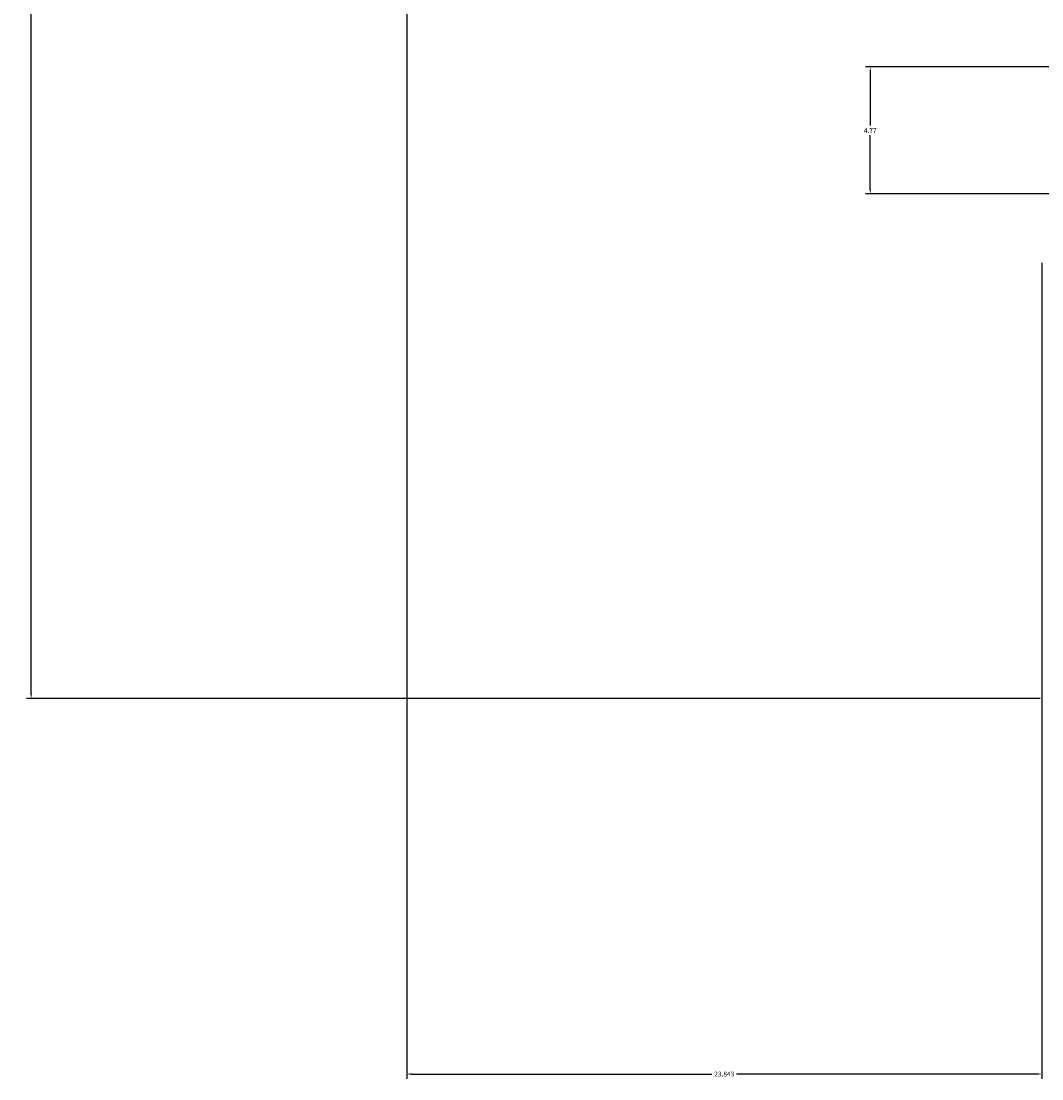
# Model space of a CAD drawing. Units: millimetres. Extents: x -8 to 285, y 5 to 221.
# Tile 1 of 30: x -8 to 31, y 5 to 45. Entities that reach past the tile are written whole.
import ezdxf

# ---------------------------------------------------------------- set-up
doc = ezdxf.new("R2010")
doc.units = ezdxf.units.MM
doc.layers.add('A-ANNO-DIMS', color=2, linetype='Continuous', lineweight=18)
doc.styles.get("Standard").update_dxf_attribs({"font": 'arial.ttf'})
doc.dimstyles.get("Standard").update_dxf_attribs({"dimtxt": 0.18, "dimasz": 0.18, "dimexe": 0.18, "dimexo": 0.0625, "dimgap": 0.09, "dimtad": 0, "dimtih": 1, "dimtoh": 1, "dimdec": 4, "dimzin": 0, "dimdsep": 46, "dimtxsty": 'Standard', "dimcen": 0.09, "dimadec": 0, "dimazin": 0, "dimtfac": 1, "dimtdec": 4, "dimtofl": 0, "dimtmove": 0, "dimatfit": 3, "dimfxl": 1, "dimtolj": 1, "dimtzin": 0, "dimarcsym": 0})

# ---------------------------------------------------------------- blocks, each defined once
blk = doc.blocks.new('*D10')
at = {"layer": 'A-ANNO-DIMS', "color": 0, "lineweight": -2, "transparency": 16777216}
for p, q in [((145.103, 206.457), (-7.608, 206.457)), ((-7.428, 206.277), (-7.428, 113.161)), ((-7.428, 19.682), (-7.428, 112.797)), ((30.453, 19.502), (-7.608, 19.502))]:
    blk.add_line(p, q, dxfattribs=at)
at = {"layer": 'A-ANNO-DIMS', "color": 0, "transparency": 16777216}
for points in [[(-7.458, 206.277), (-7.398, 206.277), (-7.428, 206.457)], [(-7.458, 19.682), (-7.398, 19.682), (-7.428, 19.502)]]:
    blk.add_solid(points, dxfattribs=at)
at = {"layer": 'Defpoints', "color": 0, "transparency": 16777216}
for p in [(-7.428, 206.457), (145.165, 206.457), (30.516, 19.502)]:
    blk.add_point(p, dxfattribs=at)
at = {"layer": 'A-ANNO-DIMS', "color": 0, "transparency": 16777216, "insert": (-7.428, 112.979), "char_height": 0.18, "attachment_point": 5}
blk.add_mtext('\\A1;186.95', dxfattribs=at)
blk = doc.blocks.new('*D20')
at = {"layer": 'A-ANNO-DIMS', "color": 0, "lineweight": -2, "transparency": 16777216}
for p, q in [((38.112044, 43.223892), (23.894544, 43.223892)), ((24.074544, 43.043892), (24.074544, 41.018795)), ((24.074544, 38.633698), (24.074544, 40.658795)), ((38.112044, 38.453698), (23.894544, 38.453698))]:
    blk.add_line(p, q, dxfattribs=at)
at = {"layer": 'A-ANNO-DIMS', "color": 0, "transparency": 16777216}
for points in [[(24.044544, 43.043892), (24.104544, 43.043892), (24.074544, 43.223892)], [(24.044544, 38.633698), (24.104544, 38.633698), (24.074544, 38.453698)]]:
    blk.add_solid(points, dxfattribs=at)
at = {"layer": 'Defpoints', "color": 0, "transparency": 16777216}
for p in [(24.074544, 43.223892), (38.174544, 43.223892), (38.174544, 38.453698)]:
    blk.add_point(p, dxfattribs=at)
at = {"layer": 'A-ANNO-DIMS', "color": 0, "transparency": 16777216, "insert": (24.074544, 40.838795), "char_height": 0.18, "attachment_point": 5}
blk.add_mtext('\\A1;4.77', dxfattribs=at)
blk = doc.blocks.new('*D22')
at = {"layer": 'A-ANNO-DIMS', "color": 0, "lineweight": -2, "transparency": 16777216}
for p, q in [((6.672, 45.959), (6.672, 5.222)), ((30.516, 35.867), (30.516, 5.222)), ((6.852, 5.402), (18.129, 5.402)), ((30.336, 5.402), (19.059, 5.402))]:
    blk.add_line(p, q, dxfattribs=at)
at = {"layer": 'A-ANNO-DIMS', "color": 0, "transparency": 16777216}
for points in [[(6.852, 5.432), (6.852, 5.372), (6.672, 5.402)], [(30.336, 5.432), (30.336, 5.372), (30.516, 5.402)]]:
    blk.add_solid(points, dxfattribs=at)
at = {"layer": 'Defpoints', "color": 0, "transparency": 16777216}
for p in [(6.672, 46.021), (30.516, 35.929), (30.516, 5.402)]:
    blk.add_point(p, dxfattribs=at)
at = {"layer": 'A-ANNO-DIMS', "color": 0, "transparency": 16777216, "insert": (18.594, 5.402), "char_height": 0.18, "attachment_point": 5}
blk.add_mtext('\\A1;23.843', dxfattribs=at)

msp = doc.modelspace()

# ---------------------------------------------------------------- dimensions: what is measured, and where the dimension line sits
at = {"layer": 'A-ANNO-DIMS'}
for base, p1, p2, picture, middle in [((-7.4275, 206.4568), (30.516, 19.502), (145.1651, 206.4568), '*D10', (-7.4275, 112.9794)), ((24.0745, 43.2239), (38.1745, 38.4537), (38.1745, 43.2239), '*D20', (24.0745, 40.8388))]:
    dim = msp.add_linear_dim(base=base, p1=p1, p2=p2, angle=90, dimstyle='Standard', override={"dimdec": 2, "dimlfac": 1, "dimrnd": 0, "dimzin": 0, "dimdsep": 46, "dimlunit": 2}, dxfattribs=at)
    dim.commit()
    dim.dimension.update_dxf_attribs({"geometry": picture, "text_midpoint": middle})
dim = msp.add_linear_dim(base=(30.51597, 5.40199), p1=(6.67248, 46.02115), p2=(30.51597, 35.92922), dimstyle='Standard', override={"dimdec": 3, "dimlfac": 1, "dimrnd": 0, "dimzin": 0, "dimdsep": 46, "dimlunit": 2}, dxfattribs=at)
dim.commit()
dim.dimension.update_dxf_attribs({"geometry": '*D22', "text_midpoint": (18.59423, 5.40199)})

doc.saveas('drawing.dxf')
